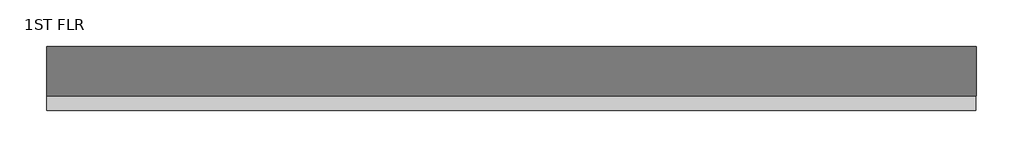
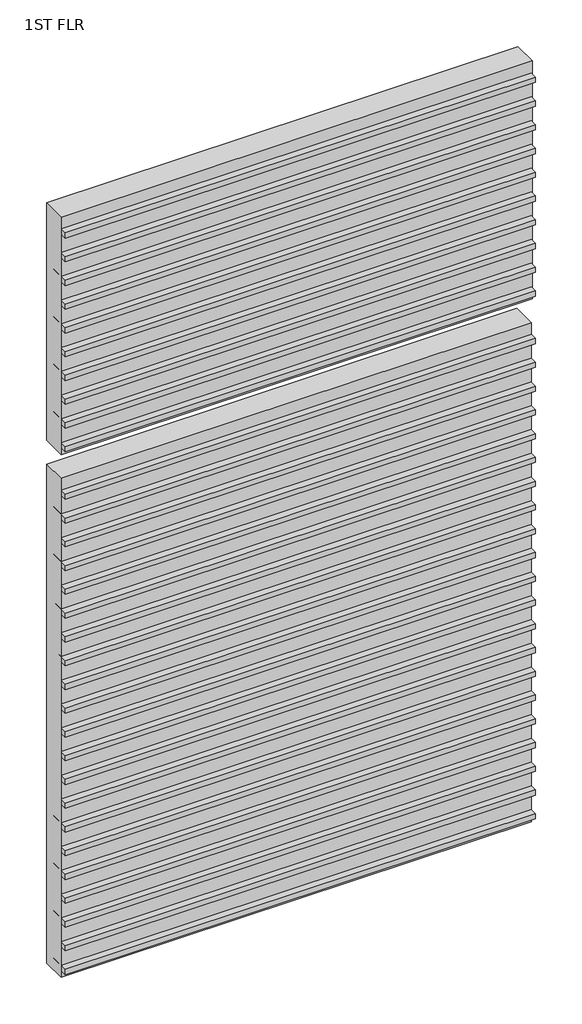
# One storey: 2 proxies.
"""IFC4 building model written with IfcOpenShell, lengths in millimetres."""

from ifc_helpers import new_model, si_unit, origin, place, context, project, spatial, transform, mapped, element, save
from components import generic_models_10_generic_models_10_37b285cf, generic_models_9_generic_models_9_38eb4f00

model = new_model("IFC4")

# Units and contexts
model_context = context("Model", 3, world=origin())
ifc_project = project(units=[si_unit("LENGTHUNIT", "METRE", prefix="MILLI")], contexts=[model_context])

# Site, building, storey
site = spatial("IfcSite", under=ifc_project)
building = spatial("IfcBuilding", under=site)
storey = spatial("IfcBuildingStorey", under=building, Name="1ST FLR", Elevation=3200.4)

# Proxies
placement = place(None, origin())
generic_models_10_generic_models_10_shape = generic_models_10_generic_models_10_37b285cf(model_context)
element("IfcBuildingElementProxy", 1, Name="Generic Models 10 : Generic Models 10", ObjectType="Generic Models 10 : Generic Models 10", at=placement, inside=storey, context=model_context, shape_type="MappedRepresentation", body=[
    mapped(generic_models_10_generic_models_10_shape, transform((0.0, 0.0, 0.0), x_axis=(1.0, 0.0, 0.0), y_axis=(0.0, 1.0, 0.0), z_axis=(0.0, 0.0, 1.0))),
])
generic_models_9_generic_models_9_shape = generic_models_9_generic_models_9_38eb4f00(model_context)
element("IfcBuildingElementProxy", 2, Name="Generic Models 9 : Generic Models 9", ObjectType="Generic Models 9 : Generic Models 9", at=placement, inside=storey, context=model_context, shape_type="MappedRepresentation", body=[
    mapped(generic_models_9_generic_models_9_shape, transform((0.0, 0.0, 0.0), x_axis=(1.0, 0.0, 0.0), y_axis=(0.0, 1.0, 0.0), z_axis=(0.0, 0.0, 1.0))),
])

save(model, "model.ifc")

# Revit data of these elements
# Element 1 (IfcBuildingElementProxy, "Generic Models 10 : Generic Models 10")
#   Phase Created = New Construction
# Element 2 (IfcBuildingElementProxy, "Generic Models 9 : Generic Models 9")
#   Phase Created = New Construction
